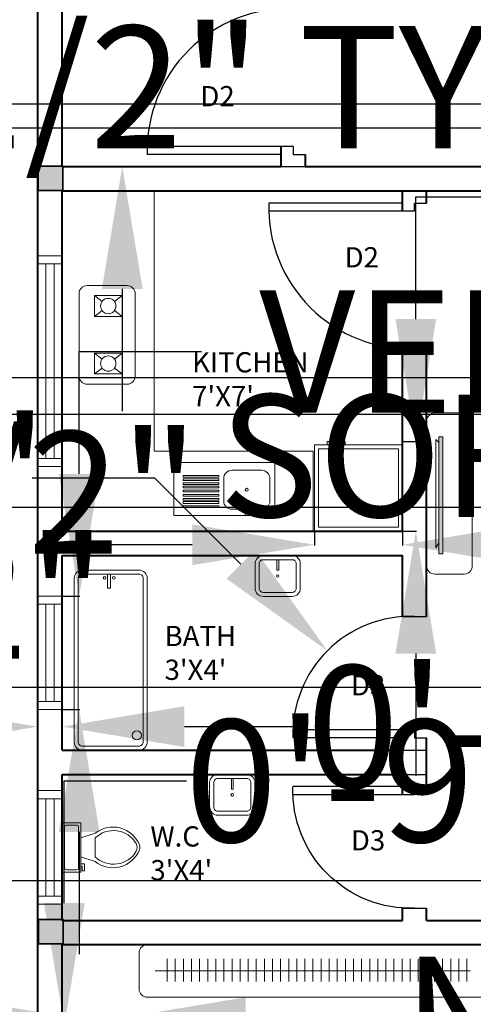
# Model space of a CAD drawing. Units: inches. Extents: x 7323 to 9737, y 2037 to 3322.
# Tile 3 of 19: x 8647 to 8759, y 2297 to 2540. Entities that reach past the tile are written whole.
import ezdxf

# ---------------------------------------------------------------- set-up
doc = ezdxf.new("R2010")
doc.units = ezdxf.units.IN
doc.header["$MEASUREMENT"] = 0
for name, color, linetype, lineweight in [('A-ANNO-DIMS', 2, 'Continuous', 18), ('A-ANNO-TEXT', 7, 'Continuous', 25), ('A-AREA-IDEN', 7, 'Continuous', 18), ('A-COLS', 1, 'Continuous', 35), ('A-DOOR', 4, 'Continuous', 25), ('A-EQPM', 9, 'Continuous', 18), ('A-FLOR-CASE', 9, 'Continuous', 20), ('A-FLOR-CASE-PATT', 8, 'Continuous', 13), ('A-FLOR-FIXT', 9, 'Continuous', 18), ('A-FURN', 8, 'Continuous', 18), ('A-FURN-PATT', 252, 'Continuous', 13), ('A-GLAZ', 4, 'Continuous', 18), ('A-WALL', 7, 'Continuous', 40)]:
    doc.layers.add(name, color=color, linetype=linetype, lineweight=lineweight)
doc.layers.add('A-COLS-PATT', color=18, linetype='Continuous', lineweight=13, true_color=0x000000)
doc.styles.get("Standard").update_dxf_attribs({"font": 'arial.ttf'})
doc.dimstyles.get("Standard").update_dxf_attribs({"dimtxt": 30.18, "dimasz": 30.18, "dimexe": 0.18, "dimexo": 0.0625, "dimgap": 0.09, "dimtad": 0, "dimtih": 1, "dimtoh": 1, "dimdec": 0, "dimzin": 0, "dimdsep": 46, "dimlunit": 3, "dimtxsty": 'Standard', "dimcen": 0.09, "dimadec": 0, "dimazin": 0, "dimtfac": 1, "dimtdec": 0, "dimtofl": 0, "dimtmove": 0, "dimatfit": 3, "dimfxl": 1, "dimtolj": 1, "dimtzin": 0, "dimarcsym": 0})

# ---------------------------------------------------------------- blocks, each defined once
blk = doc.blocks.new('*U2')
for p, q in [((9.5, -6), (9.5, -2)), ((-8, -8.5), (-8, -8)), ((-7, -8), (-7, -9.5)), ((-4, -8), (-6, -14)), ((4, -8), (6, -14)), ((-10, -8.5), (-8, -8.5)), ((-10, -9.5), (-10, -8.5)), ((-7, -9.5), (-10, -9.5)), ((4, -14), (-4, -14))]:
    blk.add_line(p, q)
blk.add_lwpolyline([(10.5, -8), (10.5, 0), (-10.5, 0), (-10.5, -8)], close=True)
for points in [[(-9.5, -2), (-9.5, -6)], [(8.5, -1), (-8.5, -1)], [(-8.5, -7), (8.5, -7)]]:
    blk.add_lwpolyline(points)
for centre, radius, start, end in [((-8.62, -1.88), 0.884, 81.8699, 188.1301), ((8.62, -1.88), 0.884, 351.8699, 98.1301), ((-8.62, -6.12), 0.884, 171.8699, 278.1301), ((8.62, -6.12), 0.884, 261.8699, 8.1301), ((3.52, -21.58), 12.17, 141.4691, 247.9714), ((4.2, -21.82), 11.33, 136.3677, 238.9468), ((-3.52, -21.58), 12.17, 292.0284, 38.5307), ((-4.2, -21.82), 11.33, 301.053, 43.6321), ((0, -27.88), 4, 245.7318, 294.2682), ((0, -29), 4, 254.8605, 285.1395)]:
    blk.add_arc(centre, radius, start, end)
blk = doc.blocks.new('WIN-48')
for p, q in [((0, 0), (0, 6)), ((2, 0), (2, 6)), ((50, 0), (50, 6)), ((52, 0), (52, 6)), ((2, 4), (50, 4)), ((2, 2), (50, 2))]:
    blk.add_line(p, q)
blk = doc.blocks.new('WIN-24')
for p, q in [((6, 28), (0, 28)), ((6, 26), (0, 26)), ((2, 26), (2, 2)), ((4, 26), (4, 2)), ((6, 2), (0, 2)), ((6, 0), (0, 0))]:
    blk.add_line(p, q)
blk = doc.blocks.new('DOOR-36')
for p, q in [((33.01, 39), (39.01, 39)), ((36.01, 5), (0.01, 5)), ((36.01, 5), (36.01, 3)), ((33.01, 3), (0.01, 3)), ((36.01, 3), (39.01, 3)), ((33.01, 0), (39.01, 0))]:
    blk.add_line(p, q)
blk.add_arc((35.01, 4), 35.01, 88.3634, 181.6366)
blk = doc.blocks.new('DOOR-36-KITCHEN')
for p, q in [((33.01, 36.01), (0.01, 36.01)), ((36.01, 36.01), (39.01, 36.01)), ((36.01, 34.01), (36.01, 36.01)), ((36.01, 34.01), (0.01, 34.01)), ((33.01, 0.01), (39.01, 0.01))]:
    blk.add_line(p, q)
blk.add_arc((35.01, 35.01), 35.01, 178.3634, 271.6366)
blk = doc.blocks.new('DOOR-30')
for p, q in [((27.01, 33), (33.01, 33)), ((30.01, 5), (0.01, 5)), ((30.01, 5), (30.01, 3)), ((27.01, 3), (0.01, 3)), ((30.01, 3), (33.01, 3)), ((27.01, 0), (33.01, 0))]:
    blk.add_line(p, q)
blk.add_arc((29.01, 4), 29.02, 88.0251, 181.9749)
blk = doc.blocks.new('KITCHEN-APPLIANCE')
for points in [[(3.16, 21.33), (3.16, 21.33), (7.58, 21.33), (7.58, 21.33), (7.58, 22.18), (7.58, 22.18), (3.16, 22.18), (3.16, 22.18)], [(21.71, 0), (21.71, 0), (0, 0), (0, 0), (0, 21.33), (0, 21.33), (21.71, 21.33), (21.71, 21.33)], [(20.71, 1), (1, 1), (1, 20.33), (20.71, 20.33)]]:
    blk.add_lwpolyline(points, close=True)
blk = doc.blocks.new('COUNTER-L')
for p, q in [((0, 84), (0, 19.81)), ((0, 19.81), (39.33, 19.81)), ((39.33, 19.81), (39.33, 0))]:
    blk.add_line(p, q)
blk = doc.blocks.new('BASIN-WALL-MOUNT')
for points in [[(0, 8.06, -0.414214), (2, 10.06), (9.16, 10.06, -0.414214), (11.16, 8.06), (11.16, 2, -0.414214), (9.16, 0), (2, 0, -0.414214), (0, 2)], [(1, 8.06, -0.414214), (2, 9.06), (9.16, 9.06, -0.414214), (10.16, 8.06), (10.16, 2, -0.414214), (9.16, 1), (2, 1, -0.414214), (1, 2)]]:
    blk.add_lwpolyline(points, format="xyb", close=True)
blk.add_lwpolyline([(5.83, 9.06), (5.83, 9.06), (5.37, 9.06), (5.37, 9.06), (5.37, 6.45), (5.37, 6.45), (5.83, 6.45), (5.83, 6.45)], close=True)
blk.add_circle((5.58, 5.03), 0.311)
blk = doc.blocks.new('COL-PLAN-6IN')
blk.add_lwpolyline([(0, 6), (0, 6), (6.06, 6), (6.06, 6), (6.06, 0), (6.06, 0), (0, 0), (0, 0)], close=True)
blk = doc.blocks.new('*D39')
at = {"layer": 'A-ANNO-DIMS', "color": 0, "lineweight": -2, "transparency": 16777216}
for p, q in [((8647.94, 2549.03), (8617.76, 2549.03)), ((8678.12, 2543.2), (8678.12, 2549.21)), ((8717.39, 2543.2), (8717.39, 2549.21)), ((8747.57, 2549.03), (8777.75, 2549.03))]:
    blk.add_line(p, q, dxfattribs=at)
at = {"layer": 'A-ANNO-DIMS', "color": 0, "transparency": 16777216}
for points in [[(8647.94, 2554.06), (8647.94, 2544), (8678.12, 2549.03)], [(8747.57, 2554.06), (8747.57, 2544), (8717.39, 2549.03)]]:
    blk.add_solid(points, dxfattribs=at)
at = {"layer": 'Defpoints', "color": 0, "transparency": 16777216}
for p in [(8717.39, 2549.03), (8678.12, 2543.14), (8717.39, 2543.14)]:
    blk.add_point(p, dxfattribs=at)
at = {"layer": 'A-ANNO-DIMS', "color": 0, "transparency": 16777216, "insert": (9057.19, 2549.03), "char_height": 30.18, "attachment_point": 5}
blk.add_mtext('\\A1;SINGLE DOOR 3\'-3 1/2" TYP.', dxfattribs=at)
blk = doc.blocks.new('*D40')
at = {"layer": 'A-ANNO-DIMS', "color": 0, "lineweight": -2, "transparency": 16777216}
for p, q in [((8672.23, 2573.32), (8672.23, 2603.5)), ((8678.06, 2543.14), (8672.05, 2543.14)), ((8678.06, 2503.86), (8672.05, 2503.86)), ((8672.23, 2473.68), (8672.23, 2443.5))]:
    blk.add_line(p, q, dxfattribs=at)
at = {"layer": 'A-ANNO-DIMS', "color": 0, "transparency": 16777216}
for points in [[(8667.2, 2573.32), (8677.26, 2573.32), (8672.23, 2543.14)], [(8667.2, 2473.68), (8677.26, 2473.68), (8672.23, 2503.86)]]:
    blk.add_solid(points, dxfattribs=at)
at = {"layer": 'Defpoints', "color": 0, "transparency": 16777216}
for p in [(8672.23, 2543.14), (8678.12, 2543.14), (8678.12, 2503.86)]:
    blk.add_point(p, dxfattribs=at)
at = {"layer": 'A-ANNO-DIMS', "color": 0, "transparency": 16777216, "insert": (8672.23, 2523.5), "char_height": 30.18, "attachment_point": 5}
blk.add_mtext('\\A1;3\'-3 1/2" TYP.', dxfattribs=at)
blk = doc.blocks.new('*D41')
at = {"layer": 'A-ANNO-DIMS', "color": 0, "lineweight": -2, "transparency": 16777216}
for p, q in [((8661.59, 2428.04), (8661.59, 2458.22)), ((8661.59, 2458.22), (8691.77, 2458.22)), ((8657.46, 2397.86), (8661.77, 2397.86)), ((8657.46, 2369.86), (8661.77, 2369.86)), ((8661.59, 2339.68), (8661.59, 2309.5))]:
    blk.add_line(p, q, dxfattribs=at)
at = {"layer": 'A-ANNO-DIMS', "color": 0, "transparency": 16777216}
for points in [[(8656.56, 2428.04), (8666.62, 2428.04), (8661.59, 2397.86)], [(8656.56, 2339.68), (8666.62, 2339.68), (8661.59, 2369.86)]]:
    blk.add_solid(points, dxfattribs=at)
at = {"layer": 'Defpoints', "color": 0, "transparency": 16777216}
for p in [(8657.39, 2397.86), (8661.59, 2397.86), (8657.39, 2369.86)]:
    blk.add_point(p, dxfattribs=at)
at = {"layer": 'A-ANNO-DIMS', "color": 0, "transparency": 16777216, "insert": (8945.06, 2458.22), "char_height": 30.18, "attachment_point": 5}
blk.add_mtext('\\A1;VENT WINDOW 2\'-4" TYP.', dxfattribs=at)
blk = doc.blocks.new('*D42')
at = {"layer": 'A-ANNO-DIMS', "color": 0, "lineweight": -2, "transparency": 16777216}
for p, q in [((8651.39, 2369.8), (8651.39, 2365.48)), ((8657.39, 2369.8), (8657.39, 2365.48)), ((8621.21, 2365.66), (8591.03, 2365.66)), ((8687.57, 2365.66), (8717.75, 2365.66))]:
    blk.add_line(p, q, dxfattribs=at)
at = {"layer": 'A-ANNO-DIMS', "color": 0, "transparency": 16777216}
for points in [[(8621.21, 2370.69), (8621.21, 2360.63), (8651.39, 2365.66)], [(8687.57, 2370.69), (8687.57, 2360.63), (8657.39, 2365.66)]]:
    blk.add_solid(points, dxfattribs=at)
at = {"layer": 'Defpoints', "color": 0, "transparency": 16777216}
for p in [(8651.39, 2369.86), (8657.39, 2369.86), (8657.39, 2365.66)]:
    blk.add_point(p, dxfattribs=at)
at = {"layer": 'A-ANNO-DIMS', "color": 0, "transparency": 16777216, "insert": (8809.82, 2365.66), "char_height": 30.18, "attachment_point": 5}
blk.add_mtext('\\A1;0\'-6" TYP.', dxfattribs=at)
blk = doc.blocks.new('*D63')
at = {"layer": 'A-ANNO-DIMS', "color": 0, "lineweight": -2, "transparency": 16777216}
for p, q in [((8744.72, 2466.22), (8744.72, 2496.4)), ((8744.72, 2496.4), (8774.9, 2496.4)), ((8741.46, 2436.04), (8744.9, 2436.04)), ((8741.46, 2413.86), (8744.9, 2413.86)), ((8744.72, 2383.68), (8744.72, 2353.5))]:
    blk.add_line(p, q, dxfattribs=at)
at = {"layer": 'A-ANNO-DIMS', "color": 0, "transparency": 16777216}
for points in [[(8739.69, 2466.22), (8749.75, 2466.22), (8744.72, 2436.04)], [(8739.69, 2383.68), (8749.75, 2383.68), (8744.72, 2413.86)]]:
    blk.add_solid(points, dxfattribs=at)
at = {"layer": 'Defpoints', "color": 0, "transparency": 16777216}
for p in [(8741.39, 2436.04), (8744.72, 2436.04), (8741.39, 2413.86)]:
    blk.add_point(p, dxfattribs=at)
at = {"layer": 'A-ANNO-DIMS', "color": 0, "transparency": 16777216, "insert": (9003.76, 2496.4), "char_height": 30.18, "attachment_point": 5}
blk.add_mtext('\\A1;APPLIANCE 1\'-10" TYP.', dxfattribs=at)
blk = doc.blocks.new('*D64')
at = {"layer": 'A-ANNO-DIMS', "color": 0, "lineweight": -2, "transparency": 16777216}
for p, q in [((8719.69, 2413.8), (8719.69, 2410.36)), ((8741.39, 2413.8), (8741.39, 2410.36)), ((8689.51, 2410.54), (8659.33, 2410.54)), ((8771.57, 2410.54), (8801.75, 2410.54))]:
    blk.add_line(p, q, dxfattribs=at)
at = {"layer": 'A-ANNO-DIMS', "color": 0, "transparency": 16777216}
for points in [[(8689.51, 2415.57), (8689.51, 2405.51), (8719.69, 2410.54)], [(8771.57, 2415.57), (8771.57, 2405.51), (8741.39, 2410.54)]]:
    blk.add_solid(points, dxfattribs=at)
at = {"layer": 'Defpoints', "color": 0, "transparency": 16777216}
for p in [(8719.69, 2413.86), (8741.39, 2413.86), (8741.39, 2410.54)]:
    blk.add_point(p, dxfattribs=at)
at = {"layer": 'A-ANNO-DIMS', "color": 0, "transparency": 16777216, "insert": (8927.57, 2410.54), "char_height": 30.18, "attachment_point": 5}
blk.add_mtext('\\A1;1\'-9 1/2" TYP.', dxfattribs=at)
blk = doc.blocks.new('*D71')
at = {"layer": 'A-ANNO-DIMS', "color": 0, "lineweight": -2, "transparency": 16777216}
for p, q in [((8891.18, 2486.02), (8891.18, 2516.2)), ((8884.24, 2455.84), (8891.36, 2455.84)), ((8884.24, 2409.18), (8891.36, 2409.18)), ((8891.18, 2379), (8891.18, 2348.82))]:
    blk.add_line(p, q, dxfattribs=at)
at = {"layer": 'A-ANNO-DIMS', "color": 0, "transparency": 16777216}
for points in [[(8886.15, 2486.02), (8896.21, 2486.02), (8891.18, 2455.84)], [(8886.15, 2379), (8896.21, 2379), (8891.18, 2409.18)]]:
    blk.add_solid(points, dxfattribs=at)
at = {"layer": 'Defpoints', "color": 0, "transparency": 16777216}
for p in [(8884.18, 2455.84), (8891.18, 2455.84), (8884.18, 2409.18)]:
    blk.add_point(p, dxfattribs=at)
at = {"layer": 'A-ANNO-DIMS', "color": 0, "transparency": 16777216, "insert": (8891.18, 2432.51), "char_height": 30.18, "attachment_point": 5}
blk.add_mtext('\\A1;SOFA 3\'-10 1/2" TYP.', dxfattribs=at)
blk = doc.blocks.new('*D75')
at = {"layer": 'A-ANNO-DIMS', "color": 0, "lineweight": -2, "transparency": 16777216}
for p, q in [((8629.63, 2293.84), (8599.45, 2293.84)), ((8659.81, 2292), (8659.81, 2294.02)), ((8672.52, 2292), (8672.52, 2294.02)), ((8702.7, 2293.84), (8732.88, 2293.84))]:
    blk.add_line(p, q, dxfattribs=at)
at = {"layer": 'A-ANNO-DIMS', "color": 0, "transparency": 16777216}
for points in [[(8629.63, 2298.87), (8629.63, 2288.81), (8659.81, 2293.84)], [(8702.7, 2298.87), (8702.7, 2288.81), (8672.52, 2293.84)]]:
    blk.add_solid(points, dxfattribs=at)
at = {"layer": 'Defpoints', "color": 0, "transparency": 16777216}
for p in [(8672.52, 2293.84), (8659.81, 2291.93), (8672.52, 2291.93)]:
    blk.add_point(p, dxfattribs=at)
at = {"layer": 'A-ANNO-DIMS', "color": 0, "transparency": 16777216, "insert": (9002.27, 2293.84), "char_height": 30.18, "attachment_point": 5}
blk.add_mtext('\\A1;NIGHTSTAND 1\'-0 1/2" TYP.', dxfattribs=at)
blk = doc.blocks.new('*D76')
at = {"layer": 'A-ANNO-DIMS', "color": 0, "lineweight": -2, "transparency": 16777216}
for p, q in [((8657.91, 2322.11), (8657.91, 2352.29)), ((8657.91, 2352.29), (8688.09, 2352.29)), ((8659.75, 2291.93), (8657.73, 2291.93)), ((8659.75, 2282.32), (8657.73, 2282.32)), ((8657.91, 2252.14), (8657.91, 2221.96))]:
    blk.add_line(p, q, dxfattribs=at)
at = {"layer": 'A-ANNO-DIMS', "color": 0, "transparency": 16777216}
for points in [[(8652.88, 2322.11), (8662.94, 2322.11), (8657.91, 2291.93)], [(8652.88, 2252.14), (8662.94, 2252.14), (8657.91, 2282.32)]]:
    blk.add_solid(points, dxfattribs=at)
at = {"layer": 'Defpoints', "color": 0, "transparency": 16777216}
for p in [(8657.91, 2291.93), (8659.81, 2291.93), (8659.81, 2282.32)]:
    blk.add_point(p, dxfattribs=at)
at = {"layer": 'A-ANNO-DIMS', "color": 0, "transparency": 16777216, "insert": (8815.32, 2352.29), "char_height": 30.18, "attachment_point": 5}
blk.add_mtext('\\A1;0\'-9 1/2" TYP.', dxfattribs=at)
blk = doc.blocks.new('*D81')
at = {"layer": 'A-ANNO-DIMS', "color": 0, "lineweight": -2, "transparency": 16777216}
for p, q in [((8651.33, 2671.86), (8587.16, 2671.86)), ((8587.34, 2641.68), (8587.34, 2443.36)), ((8587.34, 2214.04), (8587.34, 2412.36)), ((8651.33, 2183.86), (8587.16, 2183.86))]:
    blk.add_line(p, q, dxfattribs=at)
at = {"layer": 'A-ANNO-DIMS', "color": 0, "transparency": 16777216}
for points in [[(8582.31, 2641.68), (8592.37, 2641.68), (8587.34, 2671.86)], [(8582.31, 2214.04), (8592.37, 2214.04), (8587.34, 2183.86)]]:
    blk.add_solid(points, dxfattribs=at)
at = {"layer": 'Defpoints', "color": 0, "transparency": 16777216}
for p in [(8587.34, 2671.86), (8651.39, 2671.86), (8651.39, 2183.86)]:
    blk.add_point(p, dxfattribs=at)
at = {"layer": 'A-ANNO-DIMS', "color": 0, "transparency": 16777216, "insert": (8587.34, 2427.86), "char_height": 30.18, "attachment_point": 5}
blk.add_mtext('\\A1;40\'-8"', dxfattribs=at)
blk = doc.blocks.new('*D97')
at = {"layer": 'A-ANNO-DIMS', "color": 0, "lineweight": -2, "transparency": 16777216}
for p, q in [((8813.39277, 2308.800309), (8813.39277, 2148.482809)), ((8915.39277, 2183.800309), (8915.39277, 2148.482809)), ((8783.21277, 2148.662809), (8753.03277, 2148.662809)), ((8945.57277, 2148.662809), (8975.75277, 2148.662809))]:
    blk.add_line(p, q, dxfattribs=at)
at = {"layer": 'A-ANNO-DIMS', "color": 0, "transparency": 16777216}
for points in [[(8783.21277, 2153.692809), (8783.21277, 2143.632809), (8813.39277, 2148.662809)], [(8945.57277, 2153.692809), (8945.57277, 2143.632809), (8915.39277, 2148.662809)]]:
    blk.add_solid(points, dxfattribs=at)
at = {"layer": 'Defpoints', "color": 0, "transparency": 16777216}
for p in [(8813.39277, 2308.862809), (8915.39277, 2183.862809), (8915.39277, 2148.662809)]:
    blk.add_point(p, dxfattribs=at)
at = {"layer": 'A-ANNO-DIMS', "color": 0, "transparency": 16777216, "insert": (8864.39277, 2148.662809), "char_height": 30.18, "attachment_point": 5}
blk.add_mtext('\\A1;8\'-6"', dxfattribs=at)
blk = doc.blocks.new('*D98')
at = {"layer": 'A-ANNO-DIMS', "color": 0, "lineweight": -2, "transparency": 16777216}
for p, q in [((8813.33, 2317.86), (8778.01, 2317.67)), ((8778.36, 2287.49), (8778.48, 2265.91)), ((8778.77, 2213.85), (8778.65, 2235.43)), ((8814.07, 2183.86), (8778.75, 2183.67))]:
    blk.add_line(p, q, dxfattribs=at)
at = {"layer": 'A-ANNO-DIMS', "color": 0, "transparency": 16777216}
for points in [[(8783.39, 2287.52), (8773.33, 2287.46), (8778.19, 2317.67)], [(8783.79, 2213.88), (8773.74, 2213.82), (8778.93, 2183.67)]]:
    blk.add_solid(points, dxfattribs=at)
at = {"layer": 'Defpoints', "color": 0, "transparency": 16777216}
for p in [(8778.19, 2317.67), (8813.39, 2317.86), (8814.13, 2183.86)]:
    blk.add_point(p, dxfattribs=at)
at = {"layer": 'A-ANNO-DIMS', "color": 0, "transparency": 16777216, "insert": (8778.56, 2250.67), "char_height": 30.18, "attachment_point": 5}
blk.add_mtext('\\A1;11\'-2"', dxfattribs=at)
blk = doc.blocks.new('*D100')
at = {"layer": 'A-ANNO-DIMS', "color": 0, "lineweight": -2, "transparency": 16777216}
for p, q in [((9007.88, 2687.3), (8587.16, 2687.3)), ((8587.34, 2657.12), (8587.34, 2615.8)), ((8587.34, 2543.49), (8587.34, 2584.8)), ((9008.12, 2513.31), (8587.16, 2513.31))]:
    blk.add_line(p, q, dxfattribs=at)
at = {"layer": 'A-ANNO-DIMS', "color": 0, "transparency": 16777216}
for points in [[(8582.31, 2657.12), (8592.37, 2657.12), (8587.34, 2687.3)], [(8582.31, 2543.49), (8592.37, 2543.49), (8587.34, 2513.31)]]:
    blk.add_solid(points, dxfattribs=at)
at = {"layer": 'Defpoints', "color": 0, "transparency": 16777216}
for p in [(9007.95, 2687.3), (8587.34, 2513.31), (9008.18, 2513.31)]:
    blk.add_point(p, dxfattribs=at)
at = {"layer": 'A-ANNO-DIMS', "color": 0, "transparency": 16777216, "insert": (8587.34, 2600.3), "char_height": 30.18, "attachment_point": 5}
blk.add_mtext('\\A1;14\'-6"', dxfattribs=at)
blk = doc.blocks.new('*D106')
at = {"layer": 'A-ANNO-DIMS', "color": 0, "lineweight": -2, "transparency": 16777216}
for p, q in [((9008.12, 2519.31), (8587.16, 2519.31)), ((8587.34, 2489.13), (8587.34, 2439.14)), ((8587.34, 2357.76), (8587.34, 2407.75)), ((9008.23, 2327.58), (8587.16, 2327.58))]:
    blk.add_line(p, q, dxfattribs=at)
at = {"layer": 'A-ANNO-DIMS', "color": 0, "transparency": 16777216}
for points in [[(8582.31, 2489.13), (8592.37, 2489.13), (8587.34, 2519.31)], [(8582.31, 2357.76), (8592.37, 2357.76), (8587.34, 2327.58)]]:
    blk.add_solid(points, dxfattribs=at)
at = {"layer": 'Defpoints', "color": 0, "transparency": 16777216}
for p in [(8587.34, 2519.31), (9008.18, 2519.31), (9008.29, 2327.58)]:
    blk.add_point(p, dxfattribs=at)
at = {"layer": 'A-ANNO-DIMS', "color": 0, "transparency": 16777216, "insert": (8587.34, 2423.44), "char_height": 30.18, "attachment_point": 5}
blk.add_mtext('\\A1;15\'-11 1/2"', dxfattribs=at)
blk = doc.blocks.new('*D108')
at = {"layer": 'A-ANNO-DIMS', "color": 0, "lineweight": -2, "transparency": 16777216}
for p, q in [((8587.34, 2481.93), (8587.34, 2512.11)), ((8841.54, 2451.75), (8587.16, 2451.75)), ((8839.88, 2442.71), (8587.16, 2442.71)), ((8587.34, 2412.53), (8587.34, 2382.35)), ((8587.34, 2382.35), (8557.16, 2382.35))]:
    blk.add_line(p, q, dxfattribs=at)
at = {"layer": 'A-ANNO-DIMS', "color": 0, "transparency": 16777216}
for points in [[(8582.31, 2481.93), (8592.37, 2481.93), (8587.34, 2451.75)], [(8582.31, 2412.53), (8592.37, 2412.53), (8587.34, 2442.71)]]:
    blk.add_solid(points, dxfattribs=at)
at = {"layer": 'Defpoints', "color": 0, "transparency": 16777216}
for p in [(8841.6, 2451.75), (8587.34, 2442.71), (8839.94, 2442.71)]:
    blk.add_point(p, dxfattribs=at)
at = {"layer": 'A-ANNO-DIMS', "color": 0, "transparency": 16777216, "insert": (8516.96, 2382.35), "char_height": 30.18, "attachment_point": 5}
blk.add_mtext('\\A1;0\'-9"', dxfattribs=at)
blk = doc.blocks.new('*D110')
at = {"layer": 'A-ANNO-DIMS', "color": 0, "lineweight": -2, "transparency": 16777216}
for p, q in [((8587.34, 2449.91), (8587.34, 2480.09)), ((9018.85, 2419.73), (8587.16, 2419.73)), ((9018.85, 2375.3), (8587.16, 2375.3)), ((8587.34, 2345.12), (8587.34, 2314.94))]:
    blk.add_line(p, q, dxfattribs=at)
at = {"layer": 'A-ANNO-DIMS', "color": 0, "transparency": 16777216}
for points in [[(8582.31, 2449.91), (8592.37, 2449.91), (8587.34, 2419.73)], [(8582.31, 2345.12), (8592.37, 2345.12), (8587.34, 2375.3)]]:
    blk.add_solid(points, dxfattribs=at)
at = {"layer": 'Defpoints', "color": 0, "transparency": 16777216}
for p in [(8587.34, 2419.73), (9018.91, 2419.73), (9018.91, 2375.3)]:
    blk.add_point(p, dxfattribs=at)
at = {"layer": 'A-ANNO-DIMS', "color": 0, "transparency": 16777216, "insert": (8587.34, 2397.51), "char_height": 30.18, "attachment_point": 5}
blk.add_mtext('\\A1;3\'-8 1/2"', dxfattribs=at)
blk = doc.blocks.new('*D124')
at = {"layer": 'A-ANNO-DIMS', "color": 0, "lineweight": -2, "transparency": 16777216}
for p, q in [((8752.73, 2571.2), (8782.91, 2571.2)), ((8782.91, 2571.2), (8803.63, 2549.26)), ((8848.3, 2501.86), (8848.48, 2501.86)), ((8848.39, 2501.77), (8848.39, 2501.95))]:
    blk.add_line(p, q, dxfattribs=at)
at = {"layer": 'A-ANNO-DIMS', "color": 0, "transparency": 16777216}
blk.add_solid([(8807.29, 2552.71), (8799.97, 2545.81), (8824.35, 2527.32)], dxfattribs=at)
at = {"layer": 'Defpoints', "color": 0, "transparency": 16777216}
for p in [(8824.35, 2527.32), (8848.39, 2501.86)]:
    blk.add_point(p, dxfattribs=at)
at = {"layer": 'A-ANNO-DIMS', "color": 0, "transparency": 16777216, "insert": (8653.33, 2571.2), "char_height": 30.18, "attachment_point": 5}
blk.add_mtext('\\A1;4X R2\'-11"', dxfattribs=at)
blk = doc.blocks.new('*D125')
at = {"layer": 'A-ANNO-DIMS', "color": 0, "lineweight": -2, "transparency": 16777216}
for p, q in [((8650, 2427.05), (8680.18, 2427.05)), ((8680.18, 2427.05), (8701.53, 2405.72)), ((8743.3, 2363.86), (8743.48, 2363.86)), ((8743.39, 2363.77), (8743.39, 2363.95))]:
    blk.add_line(p, q, dxfattribs=at)
at = {"layer": 'A-ANNO-DIMS', "color": 0, "transparency": 16777216}
blk.add_solid([(8705.08, 2409.27), (8697.97, 2402.16), (8722.87, 2384.38)], dxfattribs=at)
at = {"layer": 'Defpoints', "color": 0, "transparency": 16777216}
for p in [(8722.87, 2384.38), (8743.39, 2363.86)]:
    blk.add_point(p, dxfattribs=at)
at = {"layer": 'A-ANNO-DIMS', "color": 0, "transparency": 16777216, "insert": (8595.36, 2427.05), "char_height": 30.18, "attachment_point": 5}
blk.add_mtext('\\A1;R2\'-5"', dxfattribs=at)

msp = doc.modelspace()

# ---------------------------------------------------------------- hatches: boundary and pattern name
at = {"layer": 'A-COLS-PATT'}
h = msp.add_hatch(color=256, dxfattribs=at)
h.dxf.hatch_style = 1
h.paths.add_polyline_path([(8915.39, 2189.86), (8908.77, 2189.86), (8908.77, 2183.86), (8915.39, 2183.86)])
h.paths.add_polyline_path([(8657.61, 2189.86), (8651.55, 2189.86), (8651.55, 2183.86), (8657.61, 2183.86)])
h.paths.add_polyline_path([(8814.13, 2189.86), (8807.39, 2189.86), (8807.39, 2183.86), (8814.13, 2183.86)])
h.paths.add_polyline_path([(8813.39, 2317.86), (8807.36, 2317.86), (8807.36, 2311.86), (8813.39, 2311.86)])
h.paths.add_polyline_path([(8915.34, 2313.13), (8909.39, 2313.13), (8909.39, 2307.13), (8915.34, 2307.13)])
h.paths.add_polyline_path([(8657.62, 2317.86), (8657.39, 2317.86), (8657.39, 2318.08), (8651.55, 2318.08), (8651.55, 2312.08), (8657.62, 2312.08)])
h.paths.add_polyline_path([(8915.39, 2671.84), (8909.37, 2671.84), (8909.37, 2665.86), (8909.39, 2665.86), (8915.39, 2665.84)])
h.paths.add_polyline_path([(8657.59, 2671.81), (8651.52, 2671.81), (8651.52, 2665.81), (8657.39, 2665.81), (8657.39, 2665.86)])
h.paths.add_polyline_path([(8915.28, 2503.94), (8909.39, 2503.94), (8909.39, 2503.86), (8909.22, 2497.94), (8915.28, 2497.94)])
h.paths.add_polyline_path([(8657.53, 2503.86), (8657.39, 2503.86), (8651.46, 2503.96), (8651.46, 2497.96), (8657.53, 2497.96)])
h.paths.add_polyline_path([(9014.24, 2519.3), (9013.95, 2519.3), (9008.18, 2519.31), (9008.18, 2513.31), (9014.24, 2513.31)])
h.paths.add_polyline_path([(9013.95, 2687.3), (9007.95, 2687.3), (9007.95, 2681.3), (9013.95, 2681.3)])
h.paths.add_polyline_path([(9271.95, 2687.3), (9266.01, 2687.3), (9266.01, 2681.35), (9271.95, 2681.35)])
h.paths.add_polyline_path([(9271.95, 2205.3), (9265.32, 2205.3), (9265.32, 2199.3), (9271.95, 2199.3)])
h.paths.add_polyline_path([(9170.68, 2205.3), (9163.95, 2205.3), (9163.95, 2199.3), (9170.68, 2199.3)])
h.paths.add_polyline_path([(9013.95, 2205.3), (9007.95, 2205.3), (9007.95, 2199.3), (9013.95, 2199.3)])
h.paths.add_polyline_path([(9271.95, 2519.51), (9265.95, 2519.51), (9265.95, 2519.3), (9265.93, 2513.51), (9271.95, 2513.51)])
h.paths.add_polyline_path([(9271.95, 2328.64), (9265.95, 2328.64), (9265.95, 2322.64), (9271.95, 2322.64)])
h.paths.add_polyline_path([(9014.35, 2333.3), (9013.95, 2333.3), (9013.95, 2333.58), (9008.29, 2333.58), (9008.29, 2327.58), (9014.35, 2327.58)])
at = {"layer": 'A-FLOR-CASE-PATT'}
h = msp.add_hatch(dxfattribs=at)
h.set_pattern_fill('ANSI31', color=256, scale=15.99876, angle=45, style=0)
h.paths.add_polyline_path([(8683.29, 2302.77), (8757.35, 2302.77), (8757.35, 2308.33), (8683.29, 2308.33)])
at = {"layer": 'A-FURN-PATT'}
h = msp.add_hatch(color=256, dxfattribs=at)
h.dxf.hatch_style = 1
h.paths.add_polyline_path([(8751.35, 2437.2), (8750.39, 2437.2), (8750.39, 2408.31), (8751.35, 2408.31)])

# ---------------------------------------------------------------- linework, layer by layer
at = {"layer": 'A-EQPM'}
for p, q in [((8665.38, 2472.02), (8667.27, 2470.59)), ((8672.18, 2472.02), (8670.28, 2470.59)), ((8665.38, 2466.9), (8667.27, 2468.33)), ((8672.18, 2466.9), (8670.28, 2468.33)), ((8665.38, 2457.81), (8667.27, 2456.38)), ((8672.18, 2457.81), (8670.28, 2456.38)), ((8665.38, 2452.69), (8667.27, 2454.12)), ((8672.18, 2452.69), (8670.28, 2454.12))]:
    msp.add_line(p, q, dxfattribs=at)
msp.add_lwpolyline([(8661.56, 2472.49, -0.414214), (8663.56, 2474.49), (8673.44, 2474.49, -0.414214), (8675.44, 2472.49), (8675.44, 2452.17, -0.414214), (8673.44, 2450.17), (8663.56, 2450.17, -0.414214), (8661.56, 2452.17)], format="xyb", close=True, dxfattribs=at)
for points in [[(8665.38, 2472.02), (8665.38, 2472.02), (8672.18, 2472.02), (8672.18, 2472.02), (8672.18, 2466.9), (8672.18, 2466.9), (8665.38, 2466.9), (8665.38, 2466.9)], [(8665.38, 2457.81), (8665.38, 2457.81), (8672.18, 2457.81), (8672.18, 2457.81), (8672.18, 2452.69), (8672.18, 2452.69), (8665.38, 2452.69), (8665.38, 2452.69)]]:
    msp.add_lwpolyline(points, close=True, dxfattribs=at)
for centre in [(8668.78, 2469.46), (8668.78, 2455.25)]:
    msp.add_circle(centre, 1.89, dxfattribs=at)
at = {"layer": 'A-FLOR-CASE'}
msp.add_line((8680.38, 2305.43), (8758.1, 2305.43), dxfattribs=at)
msp.add_lwpolyline([(8676.4, 2300.88, 0.414214), (8678.4, 2298.88), (8761.03, 2298.88, 0.414214), (8763.03, 2300.88), (8763.03, 2309.86, 0.414214), (8761.03, 2311.86), (8678.4, 2311.86, 0.414214), (8676.4, 2309.86)], format="xyb", close=True, dxfattribs=at)
at = {"layer": 'A-FLOR-FIXT'}
for points in [[(8684.93, 2430.86), (8684.93, 2430.86), (8709.93, 2430.86), (8709.93, 2430.86), (8709.93, 2417.76), (8709.93, 2417.76), (8684.93, 2417.76), (8684.93, 2417.76)], [(8687.29, 2427.66), (8687.29, 2427.66), (8696.09, 2427.66), (8696.09, 2427.66), (8696.09, 2427.23), (8696.09, 2427.23), (8687.29, 2427.23), (8687.29, 2427.23)], [(8687.29, 2426.81), (8687.29, 2426.81), (8696.09, 2426.81), (8696.09, 2426.81), (8696.09, 2426.38), (8696.09, 2426.38), (8687.29, 2426.38), (8687.29, 2426.38)], [(8687.29, 2425.86), (8687.29, 2425.86), (8696.09, 2425.86), (8696.09, 2425.86), (8696.09, 2425.43), (8696.09, 2425.43), (8687.29, 2425.43), (8687.29, 2425.43)], [(8687.29, 2425.02), (8687.29, 2425.02), (8696.09, 2425.02), (8696.09, 2425.02), (8696.09, 2424.59), (8696.09, 2424.59), (8687.29, 2424.59), (8687.29, 2424.59)], [(8687.29, 2424.03), (8687.29, 2424.03), (8696.09, 2424.03), (8696.09, 2424.03), (8696.09, 2423.6), (8696.09, 2423.6), (8687.29, 2423.6), (8687.29, 2423.6)], [(8687.29, 2422.98), (8687.29, 2422.98), (8696.09, 2422.98), (8696.09, 2422.98), (8696.09, 2422.55), (8696.09, 2422.55), (8687.29, 2422.55), (8687.29, 2422.55)], [(8687.29, 2422), (8687.29, 2422), (8696.09, 2422), (8696.09, 2422), (8696.09, 2421.57), (8696.09, 2421.57), (8687.29, 2421.57), (8687.29, 2421.57)], [(8687.29, 2421.19), (8687.29, 2421.19), (8696.09, 2421.19), (8696.09, 2421.19), (8696.09, 2420.76), (8696.09, 2420.76), (8687.29, 2420.76), (8687.29, 2420.76)], [(8687.29, 2420.14), (8687.29, 2420.14), (8696.09, 2420.14), (8696.09, 2420.14), (8696.09, 2419.71), (8696.09, 2419.71), (8687.29, 2419.71), (8687.29, 2419.71)], [(8703.2, 2417.76), (8703.2, 2417.76), (8702.57, 2417.76), (8702.57, 2417.76), (8702.57, 2420.78), (8702.57, 2420.78), (8703.2, 2420.78), (8703.2, 2420.78)], [(8668.62, 2403.3), (8668.62, 2403.3), (8669.32, 2403.3), (8669.32, 2403.3), (8669.32, 2399.83), (8669.32, 2399.83), (8668.62, 2399.83), (8668.62, 2399.83)], [(8699.64, 2352.86), (8699.64, 2352.86), (8699.18, 2352.86), (8699.18, 2352.86), (8699.18, 2350.25), (8699.18, 2350.25), (8699.64, 2350.25), (8699.64, 2350.25)]]:
    msp.add_lwpolyline(points, close=True, dxfattribs=at)
msp.add_lwpolyline([(8702.57, 2419.32), (8699.28, 2419.32, -0.414214), (8697.28, 2421.32), (8697.28, 2426.91, -0.414214), (8699.28, 2428.91), (8706.69, 2428.91, -0.414214), (8708.69, 2426.91), (8708.69, 2421.32, -0.414214), (8706.69, 2419.32), (8703.2, 2419.32)], format="xyb", dxfattribs=at)
for points in [[(8660.36, 2402.3, -0.414214), (8662.36, 2404.3), (8676.38, 2404.3, -0.414214), (8678.38, 2402.3), (8678.38, 2361.86, -0.414214), (8676.38, 2359.86), (8662.36, 2359.86, -0.414214), (8660.36, 2361.86)], [(8661.36, 2402.3, -0.414214), (8662.36, 2403.3), (8676.38, 2403.3, -0.414214), (8677.38, 2402.3), (8677.38, 2361.86, -0.414214), (8676.38, 2360.86), (8662.36, 2360.86, -0.414214), (8661.36, 2361.86)], [(8693.81, 2351.86, -0.414214), (8695.81, 2353.86), (8702.97, 2353.86, -0.414214), (8704.97, 2351.86), (8704.97, 2345.8, -0.414214), (8702.97, 2343.8), (8695.81, 2343.8, -0.414214), (8693.81, 2345.8)], [(8694.81, 2351.86, -0.414214), (8695.81, 2352.86), (8702.97, 2352.86, -0.414214), (8703.97, 2351.86), (8703.97, 2345.8, -0.414214), (8702.97, 2344.8), (8695.81, 2344.8, -0.414214), (8694.81, 2345.8)]]:
    msp.add_lwpolyline(points, format="xyb", close=True, dxfattribs=at)
for centre, radius in [((8702.98, 2424.11), 0.364), ((8667.88, 2402.39), 0.332), ((8670.15, 2402.36), 0.332), ((8675.83, 2363.5), 1.12), ((8699.39, 2348.83), 0.311)]:
    msp.add_circle(centre, radius, dxfattribs=at)
at = {"layer": 'A-FURN'}
for p, q in [((8750.39, 2435.77), (8749.67, 2436.52)), ((8749.67, 2436.52), (8749.67, 2409.75)), ((8749.67, 2409.75), (8750.39, 2410.98))]:
    msp.add_line(p, q, dxfattribs=at)
msp.add_lwpolyline([(8747.39, 2441.06, -0.414214), (8749.39, 2443.06), (8756.65, 2443.06, -0.414214), (8758.65, 2441.06), (8758.65, 2405.31, -0.414214), (8756.65, 2403.31), (8749.39, 2403.31, -0.414214), (8747.39, 2405.31)], format="xyb", close=True, dxfattribs=at)
msp.add_lwpolyline([(8750.39, 2437.2), (8750.39, 2437.2), (8751.35, 2437.2), (8751.35, 2437.2), (8751.35, 2408.31), (8751.35, 2408.31), (8750.39, 2408.31), (8750.39, 2408.31)], close=True, dxfattribs=at)
at = {"layer": 'A-WALL'}
for p, q in [((8651.39, 2183.86), (8651.39, 2671.86)), ((8657.39, 2503.86), (8657.39, 2665.86)), ((8711.39, 2508.86), (8711.39, 2503.86)), ((8717.39, 2506.86), (8717.39, 2503.86)), ((8657.39, 2503.86), (8711.39, 2503.86)), ((8717.39, 2503.86), (8779.39, 2503.86)), ((8657.39, 2497.86), (8777.39, 2497.86)), ((8657.39, 2413.86), (8657.39, 2497.86)), ((8741.39, 2492.86), (8741.39, 2497.86)), ((8741.39, 2492.86), (8741.39, 2497.86)), ((8747.39, 2494.86), (8747.39, 2497.86)), ((8747.39, 2494.86), (8747.39, 2497.86)), ((8741.39, 2413.86), (8741.39, 2458.91)), ((8741.39, 2413.86), (8741.39, 2458.91)), ((8747.39, 2407.86), (8747.39, 2458.86)), ((8747.39, 2392.86), (8747.39, 2458.86)), ((8657.39, 2413.86), (8741.39, 2413.86)), ((8657.39, 2407.86), (8741.39, 2407.86)), ((8657.39, 2359.86), (8657.39, 2407.86)), ((8741.39, 2392.81), (8741.39, 2407.86)), ((8741.39, 2359.86), (8741.39, 2364.86)), ((8747.39, 2350.86), (8747.39, 2362.86)), ((8657.39, 2359.86), (8741.39, 2359.86)), ((8657.39, 2353.86), (8741.39, 2353.86)), ((8657.39, 2317.86), (8657.39, 2353.86)), ((8741.39, 2348.86), (8741.39, 2353.86)), ((8741.39, 2317.86), (8741.39, 2320.91)), ((8747.39, 2317.86), (8747.39, 2320.86)), ((8657.39, 2317.86), (8741.39, 2317.86)), ((8747.39, 2317.86), (8813.39, 2317.86)), ((8657.39, 2189.86), (8657.39, 2311.86)), ((8657.39, 2311.86), (8807.39, 2311.86))]:
    msp.add_line(p, q, dxfattribs=at)

# ---------------------------------------------------------------- block references
at = {"layer": 'A-COLS'}
for p in [(8651.46, 2497.96), (8651.55, 2312.08)]:
    msp.add_blockref('COL-PLAN-6IN', p, dxfattribs=at)
at = {"layer": 'A-DOOR'}
for name, p in [('DOOR-36', (8678.38, 2503.86)), ('DOOR-36-KITCHEN', (8708.38, 2458.85)), ('DOOR-30', (8714.38, 2359.86))]:
    msp.add_blockref(name, p, dxfattribs=at)
at = {"layer": 'A-DOOR', "extrusion": (0, 0, -1), "zscale": -1, "rotation": 180}
msp.add_blockref('DOOR-30', (-8714.38, 2353.86), dxfattribs=at)
at = {"layer": 'A-EQPM'}
msp.add_blockref('KITCHEN-APPLIANCE', (8719.69, 2413.86), dxfattribs=at)
at = {"layer": 'A-FLOR-CASE'}
msp.add_blockref('COUNTER-L', (8680.07, 2413.86), dxfattribs=at)
at = {"layer": 'A-FLOR-FIXT'}
msp.add_blockref('BASIN-WALL-MOUNT', (8705.03, 2397.8), dxfattribs=at)
at = {"layer": 'A-FLOR-FIXT', "xscale": 0.5808479307613652, "yscale": 0.5808479307613652, "zscale": 0.5808479307613652, "rotation": 90}
msp.add_blockref('*U2', (8657.39, 2335.86), dxfattribs=at)
at = {"layer": 'A-GLAZ', "rotation": 89.99999999999191}
msp.add_blockref('WIN-48', (8657.39, 2429.86), dxfattribs=at)
at = {"layer": 'A-GLAZ'}
for p in [(8651.39, 2369.86), (8651.39, 2321.86)]:
    msp.add_blockref('WIN-24', p, dxfattribs=at)

# ---------------------------------------------------------------- texts
at = {"layer": 'A-ANNO-TEXT', "char_height": 5, "attachment_point": 1}
for s, insert in [('D2', (8691.51, 2523.74)), ('D2', (8727.13, 2483.98)), ('D3', (8728.68, 2378.35)), ('D3', (8728.68, 2340.1))]:
    msp.add_mtext_dynamic_manual_height_columns(s, width=26.304, gutter_width=1, heights=[0], dxfattribs=dict(at, insert=insert))
at = {"layer": 'A-AREA-IDEN', "char_height": 5, "attachment_point": 1}
for s, insert in [("KITCHEN\\P7'X7'", (8689.48, 2458.07)), ("BATH\\P3'X4'", (8682.67, 2390.53)), ("W.C\\P3'X4'", (8679.17, 2341.07))]:
    msp.add_mtext_dynamic_manual_height_columns(s, width=44.1759, gutter_width=1, heights=[0], dxfattribs=dict(at, insert=insert))

# ---------------------------------------------------------------- dimensions: what is measured, and where the dimension line sits
at = {"layer": 'A-ANNO-DIMS'}
for base, p1, p2, angle, picture, middle in [((8587.34, 2513.31), (9007.95, 2687.3), (9008.18, 2513.31), 90, '*D100', (8587.34, 2600.3)), ((8587.34, 2671.86), (8651.39, 2183.86), (8651.39, 2671.86), 90, '*D81', (8587.34, 2427.86)), ((8587.34, 2519.31), (9008.29, 2327.58), (9008.18, 2519.31), 90, '*D106', (8587.34, 2423.44)), ((8587.34, 2442.71), (8841.6, 2451.75), (8839.94, 2442.71), 90, '*D108', (8516.96, 2382.35)), ((8587.34, 2419.73), (9018.91, 2375.3), (9018.91, 2419.73), 90, '*D110', (8587.34, 2397.51)), ((8778.19, 2317.67), (8814.13, 2183.86), (8813.39, 2317.86), 90.3155, '*D98', (8778.56, 2250.67))]:
    dim = msp.add_linear_dim(base=base, p1=p1, p2=p2, angle=angle, dimstyle='Standard', override={"dimdec": 1, "dimlfac": 1, "dimrnd": 0, "dimzin": 1, "dimdsep": 46, "dimlunit": 4, "dimfrac": 2}, dxfattribs=at)
    dim.commit()
    dim.dimension.update_dxf_attribs({"geometry": picture, "text_midpoint": middle})
for base, p1, p2, text, picture, middle in [((8717.39, 2549.03), (8678.12, 2543.14), (8717.39, 2543.14), 'SINGLE DOOR <> TYP.', '*D39', (9057.19, 2549.03)), ((8741.39, 2410.54), (8719.69, 2413.86), (8741.39, 2413.86), '<> TYP.', '*D64', (8927.57, 2410.54)), ((8657.39, 2365.66), (8651.39, 2369.86), (8657.39, 2369.86), '<> TYP.', '*D42', (8809.82, 2365.66)), ((8672.52, 2293.84), (8659.81, 2291.93), (8672.52, 2291.93), 'NIGHTSTAND <> TYP.', '*D75', (9002.27, 2293.84))]:
    dim = msp.add_linear_dim(base=base, p1=p1, p2=p2, text=text, dimstyle='Standard', override={"dimdec": 1, "dimlfac": 1, "dimrnd": 0, "dimzin": 1, "dimdsep": 46, "dimlunit": 4, "dimfrac": 2}, dxfattribs=at)
    dim.commit()
    dim.dimension.update_dxf_attribs({"geometry": picture, "text_midpoint": middle})
dim = msp.add_radius_dim(center=(8848.39, 2501.86), mpoint=(8824.35, 2527.32), text='4X <>', dimstyle='Standard', override={"dimdec": 1, "dimlfac": 1, "dimrnd": 0, "dimzin": 1, "dimdsep": 46, "dimlunit": 4, "dimfrac": 2}, dxfattribs=at)
dim.commit()
dim.dimension.update_dxf_attribs({"geometry": '*D124', "text_midpoint": (8653.33, 2571.2)})
for base, p1, p2, text, picture, middle in [((8672.23, 2543.14), (8678.12, 2503.86), (8678.12, 2543.14), '<> TYP.', '*D40', (8672.23, 2523.5)), ((8744.72, 2436.04), (8741.39, 2413.86), (8741.39, 2436.04), 'APPLIANCE <> TYP.', '*D63', (9003.76, 2496.4)), ((8661.59, 2397.86), (8657.39, 2369.86), (8657.39, 2397.86), 'VENT WINDOW <> TYP.', '*D41', (8945.06, 2458.22)), ((8891.18, 2455.84), (8884.18, 2409.18), (8884.18, 2455.84), 'SOFA <> TYP.', '*D71', (8891.18, 2432.51)), ((8657.91, 2291.93), (8659.81, 2282.32), (8659.81, 2291.93), '<> TYP.', '*D76', (8815.32, 2352.29))]:
    dim = msp.add_linear_dim(base=base, p1=p1, p2=p2, angle=90, text=text, dimstyle='Standard', override={"dimdec": 1, "dimlfac": 1, "dimrnd": 0, "dimzin": 1, "dimdsep": 46, "dimlunit": 4, "dimfrac": 2}, dxfattribs=at)
    dim.commit()
    dim.dimension.update_dxf_attribs({"geometry": picture, "text_midpoint": middle})
dim = msp.add_radius_dim(center=(8743.39, 2363.86), mpoint=(8722.87, 2384.38), dimstyle='Standard', override={"dimdec": 1, "dimlfac": 1, "dimrnd": 0, "dimzin": 1, "dimdsep": 46, "dimlunit": 4, "dimfrac": 2}, dxfattribs=at)
dim.commit()
dim.dimension.update_dxf_attribs({"geometry": '*D125', "text_midpoint": (8595.36, 2427.05)})
dim = msp.add_linear_dim(base=(8915.39, 2148.66), p1=(8813.39, 2308.86), p2=(8915.39, 2183.86), dimstyle='Standard', override={"dimdec": 1, "dimlfac": 1, "dimrnd": 0, "dimzin": 1, "dimdsep": 46, "dimlunit": 4, "dimfrac": 2}, dxfattribs=at)
dim.commit()
dim.dimension.update_dxf_attribs({"geometry": '*D97', "text_midpoint": (8864.39, 2148.66)})

doc.saveas('drawing.dxf')
